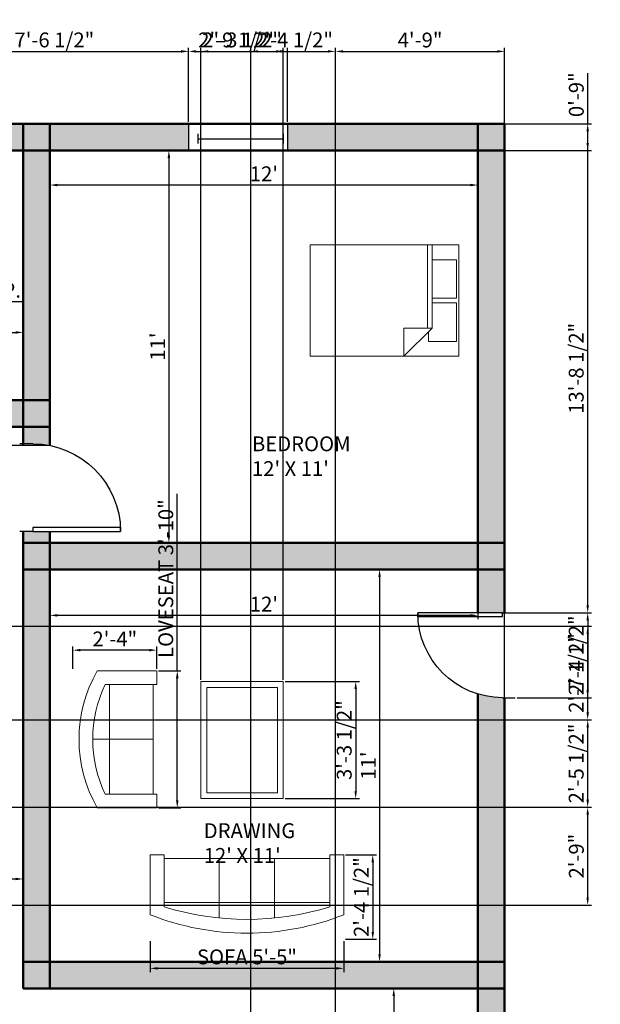
# Model space of a CAD drawing. Units: millimetres. Extents: x 3012 to 3478, y 929 to 1463.
# Tile 4 of 4: x 3283 to 3478, y 1118 to 1449. Entities that reach past the tile are written whole.
import ezdxf

# ---------------------------------------------------------------- set-up
doc = ezdxf.new("R2010")
doc.units = ezdxf.units.MM
for name, color, linetype, lineweight in [('A-ANNO-DIMS', 50, 'Continuous', 18), ('A-AREA-IDEN', 170, 'Continuous', 25), ('A-WALL-PATT', 252, 'Continuous', 13), ('doors', 130, 'Continuous', 25), ('furniture', 80, 'Continuous', 18), ('walls', 10, 'Continuous', 50), ('windows', 40, 'Continuous', 25)]:
    doc.layers.add(name, color=color, linetype=linetype, lineweight=lineweight)
doc.styles.get("Standard").update_dxf_attribs({"font": 'arial.ttf'})
doc.dimstyles.new('ISO-25', dxfattribs={"dimtxt": 5, "dimasz": 2.5, "dimexe": 1.25, "dimexo": 0.625, "dimtad": 1, "dimdec": 0, "dimlunit": 3, "dimtxsty": 'Standard', "dimcen": 2.5, "dimadec": 0, "dimazin": 0, "dimtfac": 1, "dimtdec": 0, "dimtmove": 0, "dimatfit": 3, "dimfxl": 1, "dimarcsym": 0})

# ---------------------------------------------------------------- blocks, each defined once
blk = doc.blocks.new('*U2')
for p, q in [((0, 0), (0, -6)), ((40, 0), (40, -6))]:
    blk.add_line(p, q)
blk.add_lwpolyline([(0, 0), (0, 40), (1.75, 40), (1.75, 0)], close=True)
blk.add_arc((0, 0), 40, 0, 90)
blk = doc.blocks.new('*U4')
for p, q in [((0, 4), (0, 0)), ((0, 2), (36, 2)), ((36, 4), (36, 0))]:
    blk.add_line(p, q)
blk = doc.blocks.new('Bed - Queen')
for p, q in [((0, -80.00003), (0, 0)), ((0, 0), (59.99999, 0)), ((59.99999, 0), (59.99999, -80.00003)), ((7.99999, -1.2), (28.79998, -1.2)), ((7.99999, -14.4), (7.99999, -1.2)), ((28.79998, -1.2), (28.79998, -14.4)), ((31.19999, -1.2), (51.99999, -1.2)), ((31.19999, -14.4), (31.19999, -1.2)), ((51.99999, -1.2), (51.99999, -16.4)), ((0, -14.4), (44.8, -14.4)), ((59.99999, -29.6), (44.8, -14.4)), ((44.8, -14.4), (44.8, -29.6)), ((44.8, -16.8), (0, -16.8)), ((51.99999, -16.4), (46.79936, -16.4)), ((44.8, -29.6), (59.99999, -29.6)), ((59.99999, -80.00003), (0, -80.00003))]:
    blk.add_line(p, q)
blk = doc.blocks.new('Sofa - Roundback 7 ft.')
for p, q in [((-12.00002, -32.4421), (-12.00003, -6.5971)), ((11.99997, -32.4421), (11.99998, -6.5971)), ((-36.000027, -34), (-36.000027, -11.4696)), ((35.99998, -34), (35.99998, -11.4696)), ((-35.999844, -13.3819), (35.9998, -13.3819)), ((-36.000027, -32.4421), (35.99998, -32.4421))]:
    blk.add_line(p, q)
for points in [[(-36.000027, -34), (-42.000027, -34), (-42.000027, -8)], [(41.99998, -8), (41.99998, -34), (35.99998, -34)]]:
    blk.add_lwpolyline(points)
for centre, radius, start, end in [((0, -114.25), 114.25, 68.43141, 111.5686), ((-0.00001, -127.1968), 121.1968, 72.72033, 107.2797)]:
    blk.add_arc(centre, radius, start, end)
blk = doc.blocks.new('Sofa - Roundback Loveseat 5 ft.')
for p, q in [((0, -32.44198), (0, -5.99998)), ((-24, -33.99998), (-24, -11.46958)), ((24.00004, -33.99998), (24.00004, -11.46958)), ((-23.9998, -13.38178), (23.99986, -13.38178)), ((-24, -32.44198), (24.00004, -32.44198))]:
    blk.add_line(p, q)
for points in [[(-24, -33.99998), (-30, -33.99998), (-30, -7.99998)], [(30.00004, -7.99998), (30.00004, -33.99998), (24.00004, -33.99998)]]:
    blk.add_lwpolyline(points)
for centre, radius, start, end in [((0, -60.24998), 60.24998, 60.13715, 119.8628), ((0, -61.38438), 55.38444, 64.32083, 115.6792)]:
    blk.add_arc(centre, radius, start, end)
blk = doc.blocks.new('*D14')
at = {"layer": 'A-ANNO-DIMS', "color": 0, "lineweight": -2, "transparency": 16777216}
for p, q in [((3205.21, 1344.85), (3205.21, 1345.47)), ((3284.21, 1344.85), (3284.21, 1345.47)), ((3207.71, 1344.22), (3281.71, 1344.22))]:
    blk.add_line(p, q, dxfattribs=at)
at = {"layer": 'A-ANNO-DIMS', "color": 0, "transparency": 16777216}
for points in [[(3207.71, 1344.64), (3207.71, 1343.8), (3205.21, 1344.22)], [(3281.71, 1344.64), (3281.71, 1343.8), (3284.21, 1344.22)]]:
    blk.add_solid(points, dxfattribs=at)
at = {"layer": 'Defpoints', "color": 0, "transparency": 16777216}
for p in [(3205.21, 1344.22), (3284.21, 1344.22), (3284.21, 1344.22)]:
    blk.add_point(p, dxfattribs=at)
at = {"layer": 'A-ANNO-DIMS', "color": 0, "transparency": 16777216, "insert": (3244.71, 1347.4), "char_height": 5, "attachment_point": 5}
blk.add_mtext('6\'-7"', dxfattribs=at)
blk = doc.blocks.new('*D16')
at = {"layer": 'A-ANNO-DIMS', "color": 0, "lineweight": -2, "transparency": 16777216}
for p, q in [((3327.29, 1405.44), (3334.49, 1405.44)), ((3333.24, 1402.94), (3333.24, 1275.94)), ((3327.29, 1273.44), (3334.49, 1273.44))]:
    blk.add_line(p, q, dxfattribs=at)
at = {"layer": 'A-ANNO-DIMS', "color": 0, "transparency": 16777216}
for points in [[(3332.82, 1402.94), (3333.66, 1402.94), (3333.24, 1405.44)], [(3332.82, 1275.94), (3333.66, 1275.94), (3333.24, 1273.44)]]:
    blk.add_solid(points, dxfattribs=at)
at = {"layer": 'Defpoints', "color": 0, "transparency": 16777216}
for p in [(3326.67, 1405.44), (3326.67, 1273.44), (3333.24, 1273.44)]:
    blk.add_point(p, dxfattribs=at)
at = {"layer": 'A-ANNO-DIMS', "color": 0, "transparency": 16777216, "insert": (3330.1, 1339.44), "char_height": 5, "attachment_point": 5, "rotation": 90}
blk.add_mtext("11'", dxfattribs=at)
blk = doc.blocks.new('*D23')
at = {"layer": 'A-ANNO-DIMS', "color": 0, "lineweight": -2, "transparency": 16777216}
for p, q in [((3409.52, 1123.44), (3410.15, 1123.44)), ((3408.9, 1120.94), (3408.9, 1029.94)), ((3409.52, 1027.44), (3410.15, 1027.44))]:
    blk.add_line(p, q, dxfattribs=at)
at = {"layer": 'A-ANNO-DIMS', "color": 0, "transparency": 16777216}
for points in [[(3408.48, 1120.94), (3409.31, 1120.94), (3408.9, 1123.44)], [(3408.48, 1029.94), (3409.31, 1029.94), (3408.9, 1027.44)]]:
    blk.add_solid(points, dxfattribs=at)
at = {"layer": 'Defpoints', "color": 0, "transparency": 16777216}
for p in [(3408.9, 1123.44), (3408.9, 1027.44), (3408.9, 1027.44)]:
    blk.add_point(p, dxfattribs=at)
at = {"layer": 'A-ANNO-DIMS', "color": 0, "transparency": 16777216, "insert": (3405.72, 1075.44), "char_height": 5, "attachment_point": 5, "rotation": 90}
blk.add_mtext("8'", dxfattribs=at)
blk = doc.blocks.new('*D25')
at = {"layer": 'A-ANNO-DIMS', "color": 0, "lineweight": -2, "transparency": 16777216}
for p, q in [((3125.21, 1153.8), (3125.21, 1161.53)), ((3127.71, 1160.28), (3281.71, 1160.28)), ((3284.21, 1153.8), (3284.21, 1161.53))]:
    blk.add_line(p, q, dxfattribs=at)
at = {"layer": 'A-ANNO-DIMS', "color": 0, "transparency": 16777216}
for points in [[(3127.71, 1160.7), (3127.71, 1159.86), (3125.21, 1160.28)], [(3281.71, 1160.7), (3281.71, 1159.86), (3284.21, 1160.28)]]:
    blk.add_solid(points, dxfattribs=at)
at = {"layer": 'Defpoints', "color": 0, "transparency": 16777216}
for p in [(3284.21, 1160.28), (3125.21, 1153.17), (3284.21, 1153.17)]:
    blk.add_point(p, dxfattribs=at)
at = {"layer": 'A-ANNO-DIMS', "color": 0, "transparency": 16777216, "insert": (3204.71, 1163.46), "char_height": 5, "attachment_point": 5}
blk.add_mtext('13\'-3"', dxfattribs=at)
blk = doc.blocks.new('*D27')
at = {"layer": 'A-ANNO-DIMS', "color": 0, "lineweight": -2, "transparency": 16777216}
for p, q in [((3293.21, 1394.44), (3293.21, 1395.06)), ((3437.21, 1394.44), (3437.21, 1395.06)), ((3434.71, 1393.81), (3295.71, 1393.81))]:
    blk.add_line(p, q, dxfattribs=at)
at = {"layer": 'A-ANNO-DIMS', "color": 0, "transparency": 16777216}
for points in [[(3295.71, 1394.23), (3295.71, 1393.4), (3293.21, 1393.81)], [(3434.71, 1394.23), (3434.71, 1393.4), (3437.21, 1393.81)]]:
    blk.add_solid(points, dxfattribs=at)
at = {"layer": 'Defpoints', "color": 0, "transparency": 16777216}
for p in [(3293.21, 1393.81), (3293.21, 1393.81), (3437.21, 1393.81)]:
    blk.add_point(p, dxfattribs=at)
at = {"layer": 'A-ANNO-DIMS', "color": 0, "transparency": 16777216, "insert": (3365.21, 1396.95), "char_height": 5, "attachment_point": 5}
blk.add_mtext("12'", dxfattribs=at)
blk = doc.blocks.new('*D28')
at = {"layer": 'A-ANNO-DIMS', "color": 0, "lineweight": -2, "transparency": 16777216}
for p, q in [((3397.8, 1264.44), (3405.38, 1264.44)), ((3404.13, 1261.94), (3404.13, 1134.94)), ((3397.8, 1132.44), (3405.38, 1132.44))]:
    blk.add_line(p, q, dxfattribs=at)
at = {"layer": 'A-ANNO-DIMS', "color": 0, "transparency": 16777216}
for points in [[(3403.71, 1261.94), (3404.54, 1261.94), (3404.13, 1264.44)], [(3403.71, 1134.94), (3404.54, 1134.94), (3404.13, 1132.44)]]:
    blk.add_solid(points, dxfattribs=at)
at = {"layer": 'Defpoints', "color": 0, "transparency": 16777216}
for p in [(3397.18, 1264.44), (3397.18, 1132.44), (3404.13, 1132.44)]:
    blk.add_point(p, dxfattribs=at)
at = {"layer": 'A-ANNO-DIMS', "color": 0, "transparency": 16777216, "insert": (3400.99, 1198.44), "char_height": 5, "attachment_point": 5, "rotation": 90}
blk.add_mtext("11'", dxfattribs=at)
blk = doc.blocks.new('*D29')
at = {"layer": 'A-ANNO-DIMS', "color": 0, "lineweight": -2, "transparency": 16777216}
for p, q in [((3293.21, 1256.51), (3293.21, 1247.74)), ((3437.21, 1256.51), (3437.21, 1247.74)), ((3434.71, 1248.99), (3295.71, 1248.99))]:
    blk.add_line(p, q, dxfattribs=at)
at = {"layer": 'A-ANNO-DIMS', "color": 0, "transparency": 16777216}
for points in [[(3295.71, 1249.41), (3295.71, 1248.58), (3293.21, 1248.99)], [(3434.71, 1249.41), (3434.71, 1248.58), (3437.21, 1248.99)]]:
    blk.add_solid(points, dxfattribs=at)
at = {"layer": 'Defpoints', "color": 0, "transparency": 16777216}
for p in [(3293.21, 1257.14), (3437.21, 1257.14), (3293.21, 1248.99)]:
    blk.add_point(p, dxfattribs=at)
at = {"layer": 'A-ANNO-DIMS', "color": 0, "transparency": 16777216, "insert": (3365.21, 1252.13), "char_height": 5, "attachment_point": 5}
blk.add_mtext("12'", dxfattribs=at)
blk = doc.blocks.new('*D33')
at = {"layer": 'A-ANNO-DIMS', "color": 0, "lineweight": -2, "transparency": 16777216}
for p, q in [((3222.83, 1360.33), (3222.83, 1353.34)), ((3249.8, 1360.33), (3249.8, 1353.34)), ((3225.33, 1354.59), (3247.3, 1354.59)), ((3249.8, 1354.59), (3284.11, 1354.59))]:
    blk.add_line(p, q, dxfattribs=at)
at = {"layer": 'A-ANNO-DIMS', "color": 0, "transparency": 16777216}
for points in [[(3225.33, 1355.01), (3225.33, 1354.17), (3222.83, 1354.59)], [(3247.3, 1355.01), (3247.3, 1354.17), (3249.8, 1354.59)]]:
    blk.add_solid(points, dxfattribs=at)
at = {"layer": 'Defpoints', "color": 0, "transparency": 16777216}
for p in [(3222.83, 1360.96), (3249.8, 1360.96), (3249.8, 1354.59)]:
    blk.add_point(p, dxfattribs=at)
at = {"layer": 'A-ANNO-DIMS', "color": 0, "transparency": 16777216, "insert": (3268.21, 1357.77), "char_height": 5, "attachment_point": 5}
blk.add_mtext('2\'-3" TYP.', dxfattribs=at)
blk = doc.blocks.new('*D36')
at = {"layer": 'A-ANNO-DIMS', "color": 0, "lineweight": -2, "transparency": 16777216}
for p, q in [((3326.95, 1139.34), (3326.95, 1128.95)), ((3392.07, 1139.34), (3392.07, 1128.95)), ((3389.57, 1130.2), (3329.45, 1130.2))]:
    blk.add_line(p, q, dxfattribs=at)
at = {"layer": 'A-ANNO-DIMS', "color": 0, "transparency": 16777216}
for points in [[(3329.45, 1130.62), (3329.45, 1129.78), (3326.95, 1130.2)], [(3389.57, 1130.62), (3389.57, 1129.78), (3392.07, 1130.2)]]:
    blk.add_solid(points, dxfattribs=at)
at = {"layer": 'Defpoints', "color": 0, "transparency": 16777216}
for p in [(3326.95, 1139.97), (3392.07, 1139.97), (3326.95, 1130.2)]:
    blk.add_point(p, dxfattribs=at)
at = {"layer": 'A-ANNO-DIMS', "color": 0, "transparency": 16777216, "insert": (3359.51, 1133.41), "char_height": 5, "attachment_point": 5}
blk.add_mtext('SOFA 5\'-5"', dxfattribs=at)
blk = doc.blocks.new('*D37')
at = {"layer": 'A-ANNO-DIMS', "color": 0, "lineweight": -2, "transparency": 16777216}
for p, q in [((3392.7, 1168.4), (3403.09, 1168.4)), ((3401.84, 1165.9), (3401.84, 1142.47)), ((3392.7, 1139.97), (3403.09, 1139.97))]:
    blk.add_line(p, q, dxfattribs=at)
at = {"layer": 'A-ANNO-DIMS', "color": 0, "transparency": 16777216}
for points in [[(3401.42, 1165.9), (3402.26, 1165.9), (3401.84, 1168.4)], [(3401.42, 1142.47), (3402.26, 1142.47), (3401.84, 1139.97)]]:
    blk.add_solid(points, dxfattribs=at)
at = {"layer": 'Defpoints', "color": 0, "transparency": 16777216}
for p in [(3392.07, 1168.4), (3392.07, 1139.97), (3401.84, 1139.97)]:
    blk.add_point(p, dxfattribs=at)
at = {"layer": 'A-ANNO-DIMS', "color": 0, "transparency": 16777216, "insert": (3398.63, 1154.18), "char_height": 5, "attachment_point": 5, "rotation": 90}
blk.add_mtext('2\'-4 1/2"', dxfattribs=at)
blk = doc.blocks.new('*D38')
at = {"layer": 'A-ANNO-DIMS', "color": 0, "lineweight": -2, "transparency": 16777216}
for p, q in [((3336.06, 1230.35), (3336.06, 1289.88)), ((3329.77, 1230.35), (3337.31, 1230.35)), ((3336.06, 1186.72), (3336.06, 1227.85)), ((3329.77, 1184.22), (3337.31, 1184.22))]:
    blk.add_line(p, q, dxfattribs=at)
at = {"layer": 'A-ANNO-DIMS', "color": 0, "transparency": 16777216}
for points in [[(3335.65, 1227.85), (3336.48, 1227.85), (3336.06, 1230.35)], [(3335.65, 1186.72), (3336.48, 1186.72), (3336.06, 1184.22)]]:
    blk.add_solid(points, dxfattribs=at)
at = {"layer": 'Defpoints', "color": 0, "transparency": 16777216}
for p in [(3329.14, 1230.35), (3336.06, 1230.35), (3329.14, 1184.22)]:
    blk.add_point(p, dxfattribs=at)
at = {"layer": 'A-ANNO-DIMS', "color": 0, "transparency": 16777216, "insert": (3332.85, 1261.37), "char_height": 5, "attachment_point": 5, "rotation": 90}
blk.add_mtext('LOVESEAT 3\'-10"', dxfattribs=at)
blk = doc.blocks.new('*D39')
at = {"layer": 'A-ANNO-DIMS', "color": 0, "lineweight": -2, "transparency": 16777216}
for p, q in [((3300.95, 1230.98), (3300.95, 1238.53)), ((3326.64, 1237.28), (3303.45, 1237.28)), ((3329.14, 1230.98), (3329.14, 1238.53))]:
    blk.add_line(p, q, dxfattribs=at)
at = {"layer": 'A-ANNO-DIMS', "color": 0, "transparency": 16777216}
for points in [[(3303.45, 1237.69), (3303.45, 1236.86), (3300.95, 1237.28)], [(3326.64, 1237.69), (3326.64, 1236.86), (3329.14, 1237.28)]]:
    blk.add_solid(points, dxfattribs=at)
at = {"layer": 'Defpoints', "color": 0, "transparency": 16777216}
for p in [(3300.95, 1237.28), (3300.95, 1230.35), (3329.14, 1230.35)]:
    blk.add_point(p, dxfattribs=at)
at = {"layer": 'A-ANNO-DIMS', "color": 0, "transparency": 16777216, "insert": (3315.05, 1240.41), "char_height": 5, "attachment_point": 5}
blk.add_mtext('2\'-4"', dxfattribs=at)
blk = doc.blocks.new('*D47')
at = {"layer": 'A-ANNO-DIMS', "color": 0, "lineweight": -2, "transparency": 16777216}
for p, q in [((3249.55, 1415.07), (3249.55, 1440.04)), ((3252.05, 1438.79), (3337.37, 1438.79)), ((3339.87, 1415.07), (3339.87, 1440.04))]:
    blk.add_line(p, q, dxfattribs=at)
at = {"layer": 'A-ANNO-DIMS', "color": 0, "transparency": 16777216}
for points in [[(3252.05, 1439.21), (3252.05, 1438.38), (3249.55, 1438.79)], [(3337.37, 1439.21), (3337.37, 1438.38), (3339.87, 1438.79)]]:
    blk.add_solid(points, dxfattribs=at)
at = {"layer": 'Defpoints', "color": 0, "transparency": 16777216}
for p in [(3339.87, 1438.79), (3249.55, 1414.44), (3339.87, 1414.44)]:
    blk.add_point(p, dxfattribs=at)
at = {"layer": 'A-ANNO-DIMS', "color": 0, "transparency": 16777216, "insert": (3294.71, 1442), "char_height": 5, "attachment_point": 5}
blk.add_mtext('7\'-6 1/2"', dxfattribs=at)
blk = doc.blocks.new('*D48')
at = {"layer": 'A-ANNO-DIMS', "color": 0, "lineweight": -2, "transparency": 16777216}
for p, q in [((3339.87, 1415.07), (3339.87, 1440.04)), ((3342.37, 1438.79), (3370.67, 1438.79)), ((3373.17, 1415.07), (3373.17, 1440.04))]:
    blk.add_line(p, q, dxfattribs=at)
at = {"layer": 'A-ANNO-DIMS', "color": 0, "transparency": 16777216}
for points in [[(3342.37, 1439.21), (3342.37, 1438.38), (3339.87, 1438.79)], [(3370.67, 1439.21), (3370.67, 1438.38), (3373.17, 1438.79)]]:
    blk.add_solid(points, dxfattribs=at)
at = {"layer": 'Defpoints', "color": 0, "transparency": 16777216}
for p in [(3373.17, 1438.79), (3339.87, 1414.44), (3373.17, 1414.44)]:
    blk.add_point(p, dxfattribs=at)
at = {"layer": 'A-ANNO-DIMS', "color": 0, "transparency": 16777216, "insert": (3356.52, 1442), "char_height": 5, "attachment_point": 5}
blk.add_mtext('2\'-9 1/2"', dxfattribs=at)
blk = doc.blocks.new('*D55')
at = {"layer": 'A-ANNO-DIMS', "color": 0, "lineweight": -2, "transparency": 16777216}
for p, q in [((3446.84, 1414.44), (3475.4, 1414.44)), ((3474.15, 1252.33), (3474.15, 1411.94)), ((3446.84, 1249.83), (3475.4, 1249.83))]:
    blk.add_line(p, q, dxfattribs=at)
at = {"layer": 'A-ANNO-DIMS', "color": 0, "transparency": 16777216}
for points in [[(3473.74, 1411.94), (3474.57, 1411.94), (3474.15, 1414.44)], [(3473.74, 1252.33), (3474.57, 1252.33), (3474.15, 1249.83)]]:
    blk.add_solid(points, dxfattribs=at)
at = {"layer": 'Defpoints', "color": 0, "transparency": 16777216}
for p in [(3446.21, 1414.44), (3474.15, 1414.44), (3446.21, 1249.83)]:
    blk.add_point(p, dxfattribs=at)
at = {"layer": 'A-ANNO-DIMS', "color": 0, "transparency": 16777216, "insert": (3470.94, 1332.14), "char_height": 5, "attachment_point": 5, "rotation": 90}
blk.add_mtext('13\'-8 1/2"', dxfattribs=at)
blk = doc.blocks.new('*D56')
at = {"layer": 'A-ANNO-DIMS', "color": 0, "lineweight": -2, "transparency": 16777216}
for p, q in [((3450.43, 1249.83), (3475.4, 1249.83)), ((3474.15, 1247.33), (3474.15, 1223.79)), ((3450.43, 1221.29), (3475.4, 1221.29))]:
    blk.add_line(p, q, dxfattribs=at)
at = {"layer": 'A-ANNO-DIMS', "color": 0, "transparency": 16777216}
for points in [[(3473.74, 1247.33), (3474.57, 1247.33), (3474.15, 1249.83)], [(3473.74, 1223.79), (3474.57, 1223.79), (3474.15, 1221.29)]]:
    blk.add_solid(points, dxfattribs=at)
at = {"layer": 'Defpoints', "color": 0, "transparency": 16777216}
for p in [(3449.8, 1249.83), (3449.8, 1221.29), (3474.15, 1221.29)]:
    blk.add_point(p, dxfattribs=at)
at = {"layer": 'A-ANNO-DIMS', "color": 0, "transparency": 16777216, "insert": (3470.94, 1235.56), "char_height": 5, "attachment_point": 5, "rotation": 90}
blk.add_mtext('2\'-4 1/2"', dxfattribs=at)
blk = doc.blocks.new('*D60')
at = {"layer": 'A-ANNO-DIMS', "color": 0, "lineweight": -2, "transparency": 16777216}
for p, q in [((3268.86, 1312.44), (3268.86, 1341.13)), ((3292.59, 1312.44), (3267.61, 1312.44)), ((3268.86, 1308.66), (3268.86, 1309.94)), ((3292.59, 1306.16), (3267.61, 1306.16))]:
    blk.add_line(p, q, dxfattribs=at)
at = {"layer": 'A-ANNO-DIMS', "color": 0, "transparency": 16777216}
for points in [[(3268.45, 1309.94), (3269.28, 1309.94), (3268.86, 1312.44)], [(3268.45, 1308.66), (3269.28, 1308.66), (3268.86, 1306.16)]]:
    blk.add_solid(points, dxfattribs=at)
at = {"layer": 'Defpoints', "color": 0, "transparency": 16777216}
for p in [(3268.86, 1312.44), (3293.21, 1312.44), (3293.21, 1306.16)]:
    blk.add_point(p, dxfattribs=at)
at = {"layer": 'A-ANNO-DIMS', "color": 0, "transparency": 16777216, "insert": (3265.65, 1328.04), "char_height": 5, "attachment_point": 5, "rotation": 90}
blk.add_mtext('0\'-6 1/2"', dxfattribs=at)
blk = doc.blocks.new('*D65')
at = {"layer": 'A-ANNO-DIMS', "color": 0, "lineweight": -2, "transparency": 16777216}
for p, q in [((3360.77, 1028.07), (3360.77, 1440.04)), ((3363.27, 1438.79), (3386.8, 1438.79)), ((3389.3, 1028.07), (3389.3, 1440.04))]:
    blk.add_line(p, q, dxfattribs=at)
at = {"layer": 'A-ANNO-DIMS', "color": 0, "transparency": 16777216}
for points in [[(3363.27, 1439.21), (3363.27, 1438.38), (3360.77, 1438.79)], [(3386.8, 1439.21), (3386.8, 1438.38), (3389.3, 1438.79)]]:
    blk.add_solid(points, dxfattribs=at)
at = {"layer": 'Defpoints', "color": 0, "transparency": 16777216}
for p in [(3389.3, 1438.79), (3360.77, 1027.44), (3389.3, 1027.44)]:
    blk.add_point(p, dxfattribs=at)
at = {"layer": 'A-ANNO-DIMS', "color": 0, "transparency": 16777216, "insert": (3375.03, 1442), "char_height": 5, "attachment_point": 5}
blk.add_mtext('2\'-4 1/2"', dxfattribs=at)
blk = doc.blocks.new('*D66')
at = {"layer": 'A-ANNO-DIMS', "color": 0, "lineweight": -2, "transparency": 16777216}
for p, q in [((3389.3, 1028.07), (3389.3, 1440.04)), ((3391.8, 1438.79), (3443.71, 1438.79)), ((3446.21, 1028.07), (3446.21, 1440.04))]:
    blk.add_line(p, q, dxfattribs=at)
at = {"layer": 'A-ANNO-DIMS', "color": 0, "transparency": 16777216}
for points in [[(3391.8, 1439.21), (3391.8, 1438.38), (3389.3, 1438.79)], [(3443.71, 1439.21), (3443.71, 1438.38), (3446.21, 1438.79)]]:
    blk.add_solid(points, dxfattribs=at)
at = {"layer": 'Defpoints', "color": 0, "transparency": 16777216}
for p in [(3446.21, 1438.79), (3389.3, 1027.44), (3446.21, 1027.44)]:
    blk.add_point(p, dxfattribs=at)
at = {"layer": 'A-ANNO-DIMS', "color": 0, "transparency": 16777216, "insert": (3417.76, 1441.97), "char_height": 5, "attachment_point": 5}
blk.add_mtext('4\'-9"', dxfattribs=at)
blk = doc.blocks.new('*D68')
at = {"layer": 'A-ANNO-DIMS', "color": 0, "lineweight": -2, "transparency": 16777216}
for p, q in [((3125.84, 1245.36), (3475.4, 1245.36)), ((3474.15, 1216.36), (3474.15, 1242.86)), ((3125.84, 1213.86), (3475.4, 1213.86))]:
    blk.add_line(p, q, dxfattribs=at)
at = {"layer": 'A-ANNO-DIMS', "color": 0, "transparency": 16777216}
for points in [[(3473.74, 1242.86), (3474.57, 1242.86), (3474.15, 1245.36)], [(3473.74, 1216.36), (3474.57, 1216.36), (3474.15, 1213.86)]]:
    blk.add_solid(points, dxfattribs=at)
at = {"layer": 'Defpoints', "color": 0, "transparency": 16777216}
for p in [(3125.21, 1245.36), (3474.15, 1245.36), (3125.21, 1213.86)]:
    blk.add_point(p, dxfattribs=at)
at = {"layer": 'A-ANNO-DIMS', "color": 0, "transparency": 16777216, "insert": (3470.94, 1229.61), "char_height": 5, "attachment_point": 5, "rotation": 90}
blk.add_mtext('2\'-7 1/2"', dxfattribs=at)
blk = doc.blocks.new('*D69')
at = {"layer": 'A-ANNO-DIMS', "color": 0, "lineweight": -2, "transparency": 16777216}
for p, q in [((3125.84, 1213.86), (3475.4, 1213.86)), ((3474.15, 1186.92), (3474.15, 1211.36)), ((3125.84, 1184.42), (3475.4, 1184.42))]:
    blk.add_line(p, q, dxfattribs=at)
at = {"layer": 'A-ANNO-DIMS', "color": 0, "transparency": 16777216}
for points in [[(3473.74, 1211.36), (3474.57, 1211.36), (3474.15, 1213.86)], [(3473.74, 1186.92), (3474.57, 1186.92), (3474.15, 1184.42)]]:
    blk.add_solid(points, dxfattribs=at)
at = {"layer": 'Defpoints', "color": 0, "transparency": 16777216}
for p in [(3125.21, 1213.86), (3474.15, 1213.86), (3125.21, 1184.42)]:
    blk.add_point(p, dxfattribs=at)
at = {"layer": 'A-ANNO-DIMS', "color": 0, "transparency": 16777216, "insert": (3470.94, 1199.14), "char_height": 5, "attachment_point": 5, "rotation": 90}
blk.add_mtext('2\'-5 1/2"', dxfattribs=at)
blk = doc.blocks.new('*D70')
at = {"layer": 'A-ANNO-DIMS', "color": 0, "lineweight": -2, "transparency": 16777216}
for p, q in [((3125.84, 1184.42), (3475.4, 1184.42)), ((3474.15, 1154.01), (3474.15, 1181.92)), ((3125.84, 1151.51), (3475.4, 1151.51))]:
    blk.add_line(p, q, dxfattribs=at)
at = {"layer": 'A-ANNO-DIMS', "color": 0, "transparency": 16777216}
for points in [[(3473.74, 1181.92), (3474.57, 1181.92), (3474.15, 1184.42)], [(3473.74, 1154.01), (3474.57, 1154.01), (3474.15, 1151.51)]]:
    blk.add_solid(points, dxfattribs=at)
at = {"layer": 'Defpoints', "color": 0, "transparency": 16777216}
for p in [(3125.21, 1184.42), (3474.15, 1184.42), (3125.21, 1151.51)]:
    blk.add_point(p, dxfattribs=at)
at = {"layer": 'A-ANNO-DIMS', "color": 0, "transparency": 16777216, "insert": (3470.98, 1167.97), "char_height": 5, "attachment_point": 5, "rotation": 90}
blk.add_mtext('2\'-9"', dxfattribs=at)
blk = doc.blocks.new('*D71')
at = {"layer": 'A-ANNO-DIMS', "color": 0, "lineweight": -2, "transparency": 16777216}
for p, q in [((3344.03, 1227.33), (3344.03, 1440.04)), ((3346.53, 1438.79), (3369.24, 1438.79)), ((3371.74, 1227.33), (3371.74, 1440.04))]:
    blk.add_line(p, q, dxfattribs=at)
at = {"layer": 'A-ANNO-DIMS', "color": 0, "transparency": 16777216}
for points in [[(3346.53, 1439.21), (3346.53, 1438.38), (3344.03, 1438.79)], [(3369.24, 1439.21), (3369.24, 1438.38), (3371.74, 1438.79)]]:
    blk.add_solid(points, dxfattribs=at)
at = {"layer": 'Defpoints', "color": 0, "transparency": 16777216}
for p in [(3371.74, 1438.79), (3344.03, 1226.71), (3371.74, 1226.71)]:
    blk.add_point(p, dxfattribs=at)
at = {"layer": 'A-ANNO-DIMS', "color": 0, "transparency": 16777216, "insert": (3357.88, 1442), "char_height": 5, "attachment_point": 5}
blk.add_mtext('2\'-3 1/2"', dxfattribs=at)
blk = doc.blocks.new('*D72')
at = {"layer": 'A-ANNO-DIMS', "color": 0, "lineweight": -2, "transparency": 16777216}
for p, q in [((3372.36, 1226.71), (3397.34, 1226.71)), ((3396.09, 1224.21), (3396.09, 1189.81)), ((3372.36, 1187.31), (3397.34, 1187.31))]:
    blk.add_line(p, q, dxfattribs=at)
at = {"layer": 'A-ANNO-DIMS', "color": 0, "transparency": 16777216}
for points in [[(3395.67, 1224.21), (3396.51, 1224.21), (3396.09, 1226.71)], [(3395.67, 1189.81), (3396.51, 1189.81), (3396.09, 1187.31)]]:
    blk.add_solid(points, dxfattribs=at)
at = {"layer": 'Defpoints', "color": 0, "transparency": 16777216}
for p in [(3371.74, 1226.71), (3371.74, 1187.31), (3396.09, 1187.31)]:
    blk.add_point(p, dxfattribs=at)
at = {"layer": 'A-ANNO-DIMS', "color": 0, "transparency": 16777216, "insert": (3392.88, 1207.01), "char_height": 5, "attachment_point": 5, "rotation": 90}
blk.add_mtext('3\'-3 1/2"', dxfattribs=at)
blk = doc.blocks.new('*D73')
at = {"layer": 'A-ANNO-DIMS', "color": 0, "lineweight": -2, "transparency": 16777216}
for p, q in [((3474.15, 1414.44), (3474.15, 1431.48)), ((3373.79, 1414.44), (3475.4, 1414.44)), ((3474.15, 1407.94), (3474.15, 1411.94)), ((3373.79, 1405.44), (3475.4, 1405.44))]:
    blk.add_line(p, q, dxfattribs=at)
at = {"layer": 'A-ANNO-DIMS', "color": 0, "transparency": 16777216}
for points in [[(3473.74, 1411.94), (3474.57, 1411.94), (3474.15, 1414.44)], [(3473.74, 1407.94), (3474.57, 1407.94), (3474.15, 1405.44)]]:
    blk.add_solid(points, dxfattribs=at)
at = {"layer": 'Defpoints', "color": 0, "transparency": 16777216}
for p in [(3373.17, 1414.44), (3474.15, 1414.44), (3373.17, 1405.44)]:
    blk.add_point(p, dxfattribs=at)
at = {"layer": 'A-ANNO-DIMS', "color": 0, "transparency": 16777216, "insert": (3470.98, 1424.21), "char_height": 5, "attachment_point": 5, "rotation": 90}
blk.add_mtext('0\'-9"', dxfattribs=at)

msp = doc.modelspace()

# ---------------------------------------------------------------- hatches: boundary and pattern name
at = {"layer": 'A-WALL-PATT'}
h = msp.add_hatch(color=256, dxfattribs=at)
h.dxf.hatch_style = 1
h.paths.add_polyline_path([(3052.21, 1405.44), (3043.21, 1405.44), (3043.21, 1273.44), (3052.21, 1273.44)])
h.paths.add_polyline_path([(3052.21, 1273.44), (3043.21, 1273.44), (3043.21, 1264.44), (3052.21, 1264.44)])
h.paths.add_polyline_path([(3052.21, 1264.44), (3043.21, 1264.44), (3043.21, 1132.44), (3052.21, 1132.44)])
h.paths.add_polyline_path([(3116.21, 1273.44), (3052.21, 1273.44), (3052.21, 1264.44), (3116.21, 1264.44)])
h.paths.add_polyline_path([(3125.21, 1273.44), (3116.21, 1273.44), (3116.21, 1264.44), (3125.21, 1264.44)])
h.paths.add_polyline_path([(3143.26, 1273.44), (3125.21, 1273.44), (3125.21, 1264.44), (3142.87, 1264.44), (3142.87, 1268, -0.035543)])
h.paths.add_polyline_path([(3052.21, 1414.44), (3043.21, 1414.44), (3043.21, 1405.44), (3052.21, 1405.44)])
h.paths.add_polyline_path([(3096.89, 1414.44), (3052.21, 1414.44), (3052.21, 1405.44), (3096.89, 1405.44)])
h.paths.add_polyline_path([(3196.21, 1414.44), (3129.12, 1414.44), (3129.12, 1405.44), (3196.21, 1405.44)])
h.paths.add_polyline_path([(3205.21, 1414.44), (3196.21, 1414.44), (3196.21, 1405.44), (3205.21, 1405.44)])
h.paths.add_polyline_path([(3205.21, 1405.44), (3196.21, 1405.44), (3196.21, 1321.44), (3205.21, 1321.44)])
h.paths.add_polyline_path([(3205.21, 1321.44), (3196.21, 1321.44), (3196.21, 1312.44), (3205.21, 1312.44)])
h.paths.add_polyline_path([(3205.21, 1312.44), (3196.21, 1312.44), (3196.21, 1273.44), (3205.21, 1273.44)])
h.paths.add_polyline_path([(3284.21, 1321.44), (3205.21, 1321.44), (3205.21, 1312.44), (3284.21, 1312.44)])
h.paths.add_polyline_path([(3205.21, 1273.44), (3196.21, 1273.44), (3196.21, 1264.44), (3205.21, 1264.44)])
h.paths.add_polyline_path([(3196.21, 1273.44), (3181.32, 1273.44), (3181.32, 1268), (3181.32, 1264.44), (3196.21, 1264.44)])
h.paths.add_polyline_path([(3293.21, 1405.44), (3284.21, 1405.44), (3284.21, 1321.44), (3293.21, 1321.44)])
h.paths.add_polyline_path([(3293.21, 1414.44), (3284.21, 1414.44), (3284.21, 1405.44), (3293.21, 1405.44)])
h.paths.add_polyline_path([(3284.21, 1414.44), (3249.55, 1414.44), (3249.55, 1405.44), (3284.21, 1405.44)])
h.paths.add_polyline_path([(3221.79, 1414.44), (3205.21, 1414.44), (3205.21, 1405.44), (3221.79, 1405.44)])
h.paths.add_polyline_path([(3339.87, 1414.44), (3293.21, 1414.44), (3293.21, 1405.44), (3339.87, 1405.44)])
h.paths.add_polyline_path([(3437.21, 1414.44), (3373.17, 1414.44), (3373.17, 1405.44), (3437.21, 1405.44)])
h.paths.add_polyline_path([(3446.21, 1414.44), (3437.21, 1414.44), (3437.21, 1405.44), (3446.21, 1405.44)])
h.paths.add_polyline_path([(3446.21, 1405.44), (3437.21, 1405.44), (3437.21, 1273.44), (3446.21, 1273.44)])
h.paths.add_polyline_path([(3437.21, 1273.44), (3293.21, 1273.44), (3293.21, 1264.44), (3437.21, 1264.44)])
h.paths.add_polyline_path([(3446.21, 1273.44), (3437.21, 1273.44), (3437.21, 1264.44), (3446.21, 1264.44)])
h.paths.add_polyline_path([(3446.21, 1264.44), (3437.21, 1264.44), (3437.21, 1249.83), (3445.52, 1249.83), (3446.21, 1249.83)])
h.paths.add_polyline_path([(3293.21, 1264.44), (3284.21, 1264.44), (3284.21, 1132.44), (3293.21, 1132.44)])
h.paths.add_polyline_path([(3293.21, 1273.44), (3284.21, 1273.44), (3284.21, 1264.44), (3293.21, 1264.44)])
h.paths.add_polyline_path([(3293.21, 1277.22), (3287.47, 1277.22), (3284.21, 1277.22), (3284.21, 1273.44), (3293.21, 1273.44)])
h.paths.add_polyline_path([(3125.21, 1213.86), (3116.21, 1213.86), (3116.21, 1184.42), (3125.21, 1184.42)])
h.paths.add_polyline_path([(3125.21, 1264.44), (3116.21, 1264.44), (3116.21, 1245.36), (3125.21, 1245.36)])
h.paths.add_polyline_path([(3125.21, 1151.51), (3116.21, 1151.51), (3116.21, 1132.44), (3125.21, 1132.44)])
h.paths.add_polyline_path([(3125.21, 1132.44), (3116.21, 1132.44), (3116.21, 1123.44), (3125.21, 1123.44)])
h.paths.add_polyline_path([(3151.56, 1127.56), (3151.56, 1132.44), (3125.21, 1132.44), (3125.21, 1123.44), (3151.56, 1123.44)])
h.paths.add_polyline_path([(3116.21, 1132.44), (3052.21, 1132.44), (3052.21, 1123.44), (3116.21, 1123.44)])
h.paths.add_polyline_path([(3052.21, 1132.44), (3043.21, 1132.44), (3043.21, 1123.44), (3052.21, 1123.44)])
h.paths.add_polyline_path([(3052.21, 1123.44), (3043.21, 1123.44), (3043.21, 966.44), (3052.21, 966.44)])
h.paths.add_polyline_path([(3097.57, 966.44), (3052.21, 966.44), (3052.21, 957.44), (3097.57, 957.44)])
h.paths.add_polyline_path([(3052.21, 966.44), (3043.21, 966.44), (3043.21, 957.44), (3052.21, 957.44)])
h.paths.add_polyline_path([(3215.21, 966.44), (3131.05, 966.44), (3131.05, 957.44), (3215.21, 957.44)])
h.paths.add_polyline_path([(3224.21, 966.44), (3215.21, 966.44), (3215.21, 957.44), (3224.21, 957.44)])
h.paths.add_polyline_path([(3224.21, 1004.97, -0.051409), (3218.39, 1004.37), (3215.21, 1004.37), (3215.21, 966.44), (3224.21, 966.44)])
h.paths.add_polyline_path([(3239.46, 966.44), (3224.21, 966.44), (3224.21, 957.44), (3239.46, 957.44)])
h.paths.add_polyline_path([(3344.91, 966.44), (3266.71, 966.44), (3266.71, 957.44), (3344.91, 957.44)])
h.paths.add_polyline_path([(3293.21, 1018.44), (3284.21, 1018.44), (3284.21, 966.44), (3293.21, 966.44)])
h.paths.add_polyline_path([(3293.21, 1027.44), (3284.21, 1027.44), (3284.21, 1018.44), (3293.21, 1018.44)])
h.paths.add_polyline_path([(3293.21, 1074.44), (3284.21, 1074.44), (3284.21, 1027.44), (3293.21, 1027.44)])
h.paths.add_polyline_path([(3224.21, 1074.44), (3215.21, 1074.44), (3215.21, 1032.91), (3218.39, 1032.91), (3224.21, 1032.91)])
h.paths.add_polyline_path([(3224.21, 1123.44), (3215.21, 1123.44), (3215.21, 1083.44), (3224.21, 1083.44)])
h.paths.add_polyline_path([(3224.21, 1083.44), (3215.21, 1083.44), (3215.21, 1074.44), (3224.21, 1074.44)])
h.paths.add_polyline_path([(3284.21, 1083.44), (3224.21, 1083.44), (3224.21, 1074.44), (3284.21, 1074.44)])
h.paths.add_polyline_path([(3293.21, 1083.44), (3284.21, 1083.44), (3284.21, 1074.44), (3293.21, 1074.44)])
h.paths.add_polyline_path([(3215.21, 1132.44), (3190.01, 1132.44), (3190.01, 1127.56, -0.026825), (3189.79, 1123.44), (3215.21, 1123.44)])
h.paths.add_polyline_path([(3224.21, 1132.44), (3215.21, 1132.44), (3215.21, 1123.44), (3224.21, 1123.44)])
h.paths.add_polyline_path([(3437.21, 1132.44), (3293.21, 1132.44), (3293.21, 1123.44), (3437.21, 1123.44)])
h.paths.add_polyline_path([(3293.21, 1132.44), (3284.21, 1132.44), (3284.21, 1123.44), (3293.21, 1123.44)])
h.paths.add_polyline_path([(3446.21, 1132.44), (3437.21, 1132.44), (3437.21, 1123.44), (3446.21, 1123.44)])
h.paths.add_polyline_path([(3446.21, 1123.44), (3437.21, 1123.44), (3437.21, 1027.44), (3446.21, 1027.44)])
h.paths.add_polyline_path([(3446.21, 1221.29), (3445.52, 1221.29, -0.074007), (3437.21, 1222.53), (3437.21, 1132.44), (3446.21, 1132.44)])
h.paths.add_polyline_path([(3446.21, 1018.44), (3437.21, 1018.44), (3437.21, 966.44), (3446.21, 966.44)])
h.paths.add_polyline_path([(3446.21, 1027.44), (3437.21, 1027.44), (3437.21, 1018.44), (3446.21, 1018.44)])
h.paths.add_polyline_path([(3437.21, 1027.44), (3389.3, 1027.44), (3389.3, 1025.95), (3389.3, 1018.44), (3437.21, 1018.44)])
h.paths.add_polyline_path([(3360.77, 1025.95), (3360.77, 1027.44), (3293.21, 1027.44), (3293.21, 1018.44), (3361.77, 1018.44, -0.066618)])
h.paths.add_polyline_path([(3437.21, 966.44), (3375.49, 966.44), (3375.49, 957.44), (3437.21, 957.44)])
h.paths.add_polyline_path([(3446.21, 966.44), (3437.21, 966.44), (3437.21, 957.44), (3446.21, 957.44)])
h = msp.add_hatch(color=256, dxfattribs=at)
h.dxf.hatch_style = 1
h.paths.add_polyline_path([(3293.21, 1321.44), (3284.21, 1321.44), (3284.21, 1312.44), (3293.21, 1312.44)])
h.paths.add_polyline_path([(3293.21, 1312.44), (3284.21, 1312.44), (3284.21, 1306.73), (3287.47, 1306.73, -0.049001), (3293.21, 1306.16)])

# ---------------------------------------------------------------- linework, layer by layer
at = {"layer": 'furniture'}
for points in [[(3344.03, 1226.71), (3371.74, 1226.71), (3371.74, 1187.31), (3344.03, 1187.31)], [(3346.03, 1224.71), (3369.74, 1224.71), (3369.74, 1189.31), (3346.03, 1189.31)]]:
    msp.add_lwpolyline(points, close=True, dxfattribs=at)
at = {"layer": 'walls'}
for p, q in [((3043.21, 1414.44), (3446.21, 1414.44)), ((3284.21, 1414.44), (3284.21, 1306.39)), ((3293.21, 1414.44), (3293.21, 1306.16)), ((3437.21, 1414.44), (3437.21, 1264.44)), ((3446.21, 1414.44), (3446.21, 1264.44)), ((3043.21, 1405.44), (3446.21, 1405.44)), ((3196.21, 1321.44), (3293.21, 1321.44)), ((3196.21, 1312.44), (3293.21, 1312.44)), ((3284.21, 1277.22), (3284.21, 1123.44)), ((3293.21, 1277.22), (3293.21, 1123.44)), ((3284.21, 1273.44), (3446.21, 1273.44)), ((3284.21, 1264.44), (3446.21, 1264.44)), ((3437.21, 1264.44), (3437.21, 1249.83)), ((3446.21, 1264.44), (3446.21, 1249.83)), ((3437.21, 1222.53), (3437.21, 957.44)), ((3446.21, 1221.29), (3446.21, 957.44)), ((3284.21, 1132.44), (3446.21, 1132.44)), ((3284.21, 1123.44), (3446.21, 1123.44))]:
    msp.add_line(p, q, dxfattribs=at)
at = {"layer": 'windows'}
for p, q in [((3339.87, 1414.44), (3339.87, 1405.44)), ((3373.17, 1414.44), (3373.17, 1405.44))]:
    msp.add_line(p, q, dxfattribs=at)

# ---------------------------------------------------------------- block references
at = {"layer": 'doors'}
for p, xscale, yscale, zscale, rotation in [((3287.47, 1277.22), -0.7377610176749388, 0.7377610176749388, 0.7377610176749388, 270), ((3445.52, 1249.83), -0.7134266761523853, 0.7134266761523853, 0.7134266761523853, 90.00000000000007)]:
    msp.add_blockref('*U2', p, dxfattribs=dict(at, xscale=xscale, yscale=yscale, zscale=zscale, rotation=rotation))
at = {"layer": 'furniture'}
for name, p, xscale, yscale, zscale, rotation in [('Bed - Queen', (3430.8, 1373.7), 0.625172702944318, 0.625172702944318, 0.625172702944318, 270), ('Sofa - Roundback Loveseat 5 ft.', (3303, 1207.29), 0.768952026566892, 0.768952026566892, 0.768952026566892, 90), ('Sofa - Roundback 7 ft.', (3359.51, 1142.04), 0.7752779043732473, 0.7752779043732473, 0.7752779043732473, 180)]:
    msp.add_blockref(name, p, dxfattribs=dict(at, xscale=xscale, yscale=yscale, zscale=zscale, rotation=rotation))
at = {"layer": 'windows', "xscale": 0.7972415233030418, "yscale": 0.7972415233030418, "zscale": 0.7972415233030418}
msp.add_blockref('*U4', (3342.94, 1407.81), dxfattribs=at)

# ---------------------------------------------------------------- texts
at = {"layer": 'A-AREA-IDEN', "char_height": 5, "attachment_point": 1}
for s, width, insert in [("BEDROOM \\P12' X 11'", 56.2972, (3361.19, 1309.22)), ("DRAWING \\P12' X 11'", 47.1, (3344.97, 1179.03))]:
    msp.add_mtext_dynamic_manual_height_columns(s, width=width, gutter_width=12.5, heights=[0], dxfattribs=dict(at, insert=insert))

# ---------------------------------------------------------------- dimensions: what is measured, and where the dimension line sits
at = {"layer": 'A-ANNO-DIMS'}
for base, p1, p2, override, picture, middle in [((3339.87, 1438.79), (3249.55, 1414.44), (3339.87, 1414.44), {"dimdec": 1, "dimlfac": 1, "dimrnd": 0, "dimzin": 1, "dimdsep": 46, "dimlunit": 4, "dimfrac": 2}, '*D47', (3294.71, 1442)), ((3373.17, 1438.79), (3339.87, 1414.44), (3373.17, 1414.44), {"dimdec": 1, "dimlfac": 1, "dimrnd": 0, "dimzin": 1, "dimdsep": 46, "dimlunit": 4, "dimfrac": 2}, '*D48', (3356.52, 1442)), ((3371.74, 1438.79), (3344.03, 1226.71), (3371.74, 1226.71), {"dimdec": 1, "dimlfac": 1, "dimrnd": 0, "dimzin": 1, "dimdsep": 46, "dimlunit": 4, "dimfrac": 2}, '*D71', (3357.88, 1442)), ((3389.3, 1438.79), (3360.77, 1027.44), (3389.3, 1027.44), {"dimdec": 1, "dimlfac": 1, "dimrnd": 0, "dimzin": 1, "dimdsep": 46, "dimlunit": 4, "dimfrac": 2}, '*D65', (3375.03, 1442)), ((3446.21, 1438.79), (3389.3, 1027.44), (3446.21, 1027.44), {"dimdec": 1, "dimlfac": 1, "dimrnd": 0, "dimzin": 1, "dimdsep": 46, "dimlunit": 4, "dimfrac": 2}, '*D66', (3417.76, 1441.97)), ((3293.21, 1393.81), (3437.21, 1393.81), (3293.21, 1393.81), {"dimclrd": 0, "dimclre": 0, "dimclrt": 0}, '*D27', (3365.21, 1396.95)), ((3284.21, 1344.22), (3205.21, 1344.22), (3284.21, 1344.22), {"dimclrd": 0, "dimclre": 0, "dimclrt": 0}, '*D14', (3244.71, 1347.4)), ((3293.21, 1248.99), (3437.21, 1257.14), (3293.21, 1257.14), {"dimclrd": 0, "dimclre": 0, "dimclrt": 0}, '*D29', (3365.21, 1252.13)), ((3284.21, 1160.28), (3125.21, 1153.17), (3284.21, 1153.17), {"dimclrd": 0, "dimclre": 0, "dimclrt": 0}, '*D25', (3204.71, 1163.46))]:
    dim = msp.add_linear_dim(base=base, p1=p1, p2=p2, dimstyle='ISO-25', override=override, dxfattribs=at)
    dim.commit()
    dim.dimension.update_dxf_attribs({"geometry": picture, "text_midpoint": middle})
for base, p1, p2, angle, override, picture, middle in [((3474.15, 1414.44), (3373.17, 1405.44), (3373.17, 1414.44), 90, {"dimdec": 1, "dimlfac": 1, "dimrnd": 0, "dimzin": 1, "dimdsep": 46, "dimlunit": 4, "dimfrac": 2}, '*D73', (3470.98, 1424.21)), ((3474.15, 1414.44), (3446.21, 1249.83), (3446.21, 1414.44), 90, {"dimdec": 1, "dimlfac": 1, "dimrnd": 0, "dimzin": 1, "dimdsep": 46, "dimlunit": 4, "dimfrac": 2}, '*D55', (3470.94, 1332.14)), ((3333.24, 1273.44), (3326.67, 1405.44), (3326.67, 1273.44), 90, {"dimclrd": 0, "dimclre": 0, "dimclrt": 0}, '*D16', (3330.1, 1339.44)), ((3268.86, 1312.44), (3293.21, 1306.16), (3293.21, 1312.44), 90, {"dimdec": 1, "dimlfac": 1, "dimrnd": 0, "dimzin": 1, "dimdsep": 46, "dimlunit": 4, "dimfrac": 2}, '*D60', (3265.65, 1328.04)), ((3404.13, 1132.44), (3397.18, 1264.44), (3397.18, 1132.44), 90, {"dimclrd": 0, "dimclre": 0, "dimclrt": 0}, '*D28', (3400.99, 1198.44)), ((3474.15, 1221.29), (3449.8, 1249.83), (3449.8, 1221.29), 270, {"dimdec": 1, "dimlfac": 1, "dimrnd": 0, "dimzin": 1, "dimdsep": 46, "dimlunit": 4, "dimfrac": 2}, '*D56', (3470.94, 1235.56)), ((3474.15, 1245.36), (3125.21, 1213.86), (3125.21, 1245.36), 90, {"dimdec": 1, "dimlfac": 1, "dimrnd": 0, "dimzin": 1, "dimdsep": 46, "dimlunit": 4, "dimfrac": 2}, '*D68', (3470.94, 1229.61)), ((3300.95, 1237.28), (3329.14, 1230.35), (3300.95, 1230.35), 180, {"dimdec": 1, "dimlfac": 1, "dimrnd": 0, "dimzin": 1, "dimdsep": 46, "dimlunit": 4, "dimfrac": 2}, '*D39', (3315.05, 1240.41)), ((3396.09, 1187.31), (3371.74, 1226.71), (3371.74, 1187.31), 270, {"dimdec": 1, "dimlfac": 1, "dimrnd": 0, "dimzin": 1, "dimdsep": 46, "dimlunit": 4, "dimfrac": 2}, '*D72', (3392.88, 1207.01)), ((3474.15, 1213.86), (3125.21, 1184.42), (3125.21, 1213.86), 90, {"dimdec": 1, "dimlfac": 1, "dimrnd": 0, "dimzin": 1, "dimdsep": 46, "dimlunit": 4, "dimfrac": 2}, '*D69', (3470.94, 1199.14)), ((3474.15, 1184.42), (3125.21, 1151.51), (3125.21, 1184.42), 90, {"dimdec": 1, "dimlfac": 1, "dimrnd": 0, "dimzin": 1, "dimdsep": 46, "dimlunit": 4, "dimfrac": 2}, '*D70', (3470.98, 1167.97)), ((3401.84, 1139.97), (3392.07, 1168.4), (3392.07, 1139.97), 270, {"dimdec": 1, "dimlfac": 1, "dimrnd": 0, "dimzin": 1, "dimdsep": 46, "dimlunit": 4, "dimfrac": 2}, '*D37', (3398.63, 1154.18)), ((3408.9, 1027.44), (3408.9, 1123.44), (3408.9, 1027.44), 90, {"dimclrd": 0, "dimclre": 0, "dimclrt": 0}, '*D23', (3405.72, 1075.44))]:
    dim = msp.add_linear_dim(base=base, p1=p1, p2=p2, angle=angle, dimstyle='ISO-25', override=override, dxfattribs=at)
    dim.commit()
    dim.dimension.update_dxf_attribs({"geometry": picture, "text_midpoint": middle})
dim = msp.add_linear_dim(base=(3249.8, 1354.59), p1=(3222.83, 1360.96), p2=(3249.8, 1360.96), text='<> TYP.', dimstyle='ISO-25', override={"dimdec": 1, "dimlfac": 1, "dimrnd": 0, "dimzin": 1, "dimdsep": 46, "dimlunit": 4, "dimfrac": 2}, dxfattribs=at)
dim.commit()
dim.dimension.update_dxf_attribs({"geometry": '*D33', "text_midpoint": (3268.21, 1357.77)})
for base, p1, p2, angle, text, picture, middle in [((3336.06, 1230.35), (3329.14, 1184.22), (3329.14, 1230.35), 90, 'LOVESEAT <>', '*D38', (3332.85, 1261.37)), ((3326.95, 1130.2), (3392.07, 1139.97), (3326.95, 1139.97), 180, 'SOFA <>', '*D36', (3359.51, 1133.41))]:
    dim = msp.add_linear_dim(base=base, p1=p1, p2=p2, angle=angle, text=text, dimstyle='ISO-25', override={"dimdec": 1, "dimlfac": 1, "dimrnd": 0, "dimzin": 1, "dimdsep": 46, "dimlunit": 4, "dimfrac": 2}, dxfattribs=at)
    dim.commit()
    dim.dimension.update_dxf_attribs({"geometry": picture, "text_midpoint": middle})

doc.saveas('drawing.dxf')
